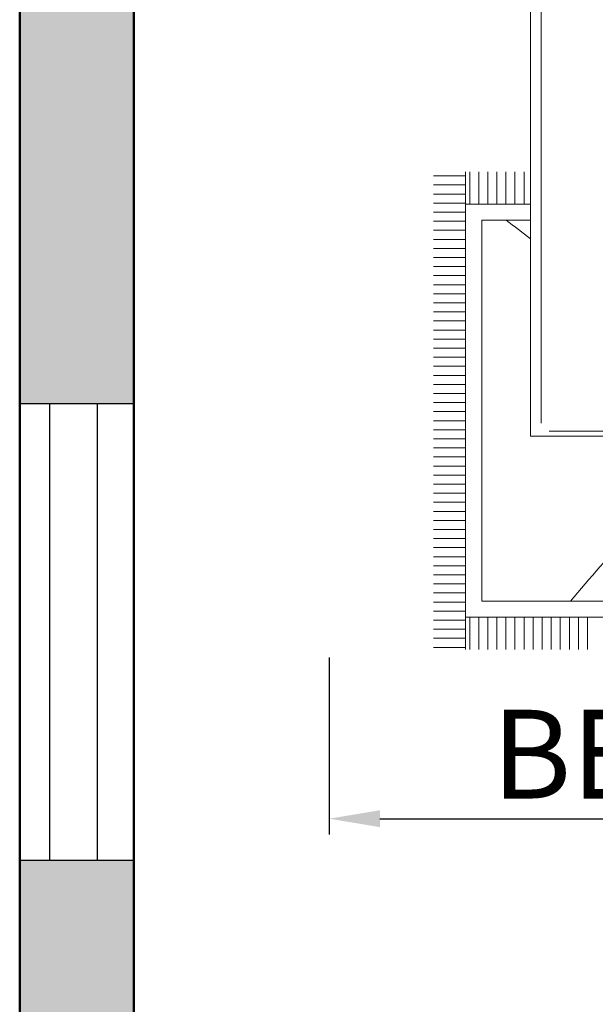
# Model space of a CAD drawing. Units: inches. Extents: x -7 to 1228, y -146 to 1091.
# Tile 8 of 88: x 60 to 105, y 375 to 453. Entities that reach past the tile are written whole.
import ezdxf

# ---------------------------------------------------------------- set-up
doc = ezdxf.new("R2010")
doc.units = ezdxf.units.IN
for name, color, linetype, lineweight in [('A-ANNO-DIMS', 2, 'Continuous', 18), ('A-FURN', 8, 'Continuous', 18), ('A-GLAZ', 175, 'Continuous', 25), ('A-WALL', 7, 'Continuous', 50), ('A-WALL-PATT', 251, 'Continuous', 13)]:
    doc.layers.add(name, color=color, linetype=linetype, lineweight=lineweight)
doc.styles.add('DIM_FONT', font='SIMPLEX.shx', dxfattribs={"width": 0.8})
doc.styles.get("Standard").update_dxf_attribs({"font": 'arial.ttf'})
doc.dimstyles.new('ISO-25', dxfattribs={"dimtxt": 7, "dimasz": 4, "dimexe": 1.25, "dimexo": 0.625, "dimtad": 1, "dimdec": 1, "dimlunit": 3, "dimtxsty": 'Standard', "dimcen": 2.5, "dimadec": 0, "dimazin": 0, "dimtfac": 1, "dimtdec": 1, "dimtmove": 1, "dimatfit": 3, "dimfxl": 1, "dimarcsym": 0})

# ---------------------------------------------------------------- blocks, each defined once
blk = doc.blocks.new('A$C4F634EDD')
for p, q in [((0.5, 0.5295), (0.5, 2.6295)), ((0.5258, 2.121), (0.5258, 0.5617)), ((0.2586, 1.1753), (0.3386, 1.1753)), ((0.3386, 0), (0.3386, 1.1852)), ((0.3486, 1.1052), (0.3486, 1.1852)), ((0.3711, 1.1052), (0.3711, 1.1852)), ((0.3936, 1.1052), (0.3936, 1.1852)), ((0.4161, 1.1052), (0.4161, 1.1852)), ((0.4386, 1.1052), (0.4386, 1.1852)), ((0.4611, 1.1052), (0.4611, 1.1852)), ((0.4836, 1.1052), (0.4836, 1.1852)), ((0.2586, 1.1528), (0.3386, 1.1528)), ((0.2586, 1.1303), (0.3386, 1.1303)), ((0.2586, 1.1078), (0.3386, 1.1078)), ((0.3386, 1.1052), (0.5, 1.1052)), ((0.2586, 1.0853), (0.3386, 1.0853)), ((0.2586, 1.0628), (0.3386, 1.0628)), ((0.3786, 1.0652), (0.5, 1.0652)), ((0.3786, 0.12), (0.3786, 1.0652)), ((0.2586, 1.0403), (0.3386, 1.0403)), ((0.2586, 1.0178), (0.3386, 1.0178)), ((0.2586, 0.9953), (0.3386, 0.9953)), ((0.2586, 0.9728), (0.3386, 0.9728)), ((0.2586, 0.9503), (0.3386, 0.9503)), ((0.2586, 0.9278), (0.3386, 0.9278)), ((0.2586, 0.9053), (0.3386, 0.9053)), ((0.2586, 0.8828), (0.3386, 0.8828)), ((0.2586, 0.8603), (0.3386, 0.8603)), ((0.2586, 0.8378), (0.3386, 0.8378)), ((0.2586, 0.8153), (0.3386, 0.8153)), ((0.2586, 0.7928), (0.3386, 0.7928)), ((0.2586, 0.7703), (0.3386, 0.7703)), ((0.2586, 0.7478), (0.3386, 0.7478)), ((0.2586, 0.7253), (0.3386, 0.7253)), ((0.2586, 0.7028), (0.3386, 0.7028)), ((0.2586, 0.6803), (0.3386, 0.6803)), ((0.2586, 0.6578), (0.3386, 0.6578)), ((0.2586, 0.6353), (0.3386, 0.6353)), ((0.2586, 0.6128), (0.3386, 0.6128)), ((0.2586, 0.5903), (0.3386, 0.5903)), ((0.2586, 0.5678), (0.3386, 0.5678)), ((0.2586, 0.5453), (0.3386, 0.5453)), ((0.5458, 0.5417), (2.2516, 0.5417)), ((0.2586, 0.5228), (0.3386, 0.5228)), ((2.3, 0.5295), (0.5, 0.5295)), ((0.2586, 0.5003), (0.3386, 0.5003)), ((0.2586, 0.4778), (0.3386, 0.4778)), ((0.2586, 0.4553), (0.3386, 0.4553)), ((0.2586, 0.4328), (0.3386, 0.4328)), ((0.2586, 0.4103), (0.3386, 0.4103)), ((0.2586, 0.3878), (0.3386, 0.3878)), ((0.2586, 0.3653), (0.3386, 0.3653)), ((0.2586, 0.3428), (0.3386, 0.3428)), ((0.2586, 0.3203), (0.3386, 0.3203)), ((0.2586, 0.2978), (0.3386, 0.2978)), ((0.2586, 0.2753), (0.3386, 0.2753)), ((0.2586, 0.2528), (0.3386, 0.2528)), ((0.2586, 0.2303), (0.3386, 0.2303)), ((0.2586, 0.2078), (0.3386, 0.2078)), ((0.2586, 0.1853), (0.3386, 0.1853)), ((0.2586, 0.1628), (0.3386, 0.1628)), ((0.2586, 0.1403), (0.3386, 0.1403)), ((0.2586, 0.1178), (0.3386, 0.1178)), ((2.4188, 0.12), (0.3786, 0.12)), ((0.2586, 0.0953), (0.3386, 0.0953)), ((2.4588, 0.08), (0.3386, 0.08)), ((0.3486, 0), (0.3486, 0.08)), ((0.3711, 0), (0.3711, 0.08)), ((0.3936, 0), (0.3936, 0.08)), ((0.4161, 0), (0.4161, 0.08)), ((0.4386, 0), (0.4386, 0.08)), ((0.4611, 0), (0.4611, 0.08)), ((0.4836, 0), (0.4836, 0.08)), ((0.5061, 0), (0.5061, 0.08)), ((0.5286, 0), (0.5286, 0.08)), ((0.5511, 0), (0.5511, 0.08)), ((0.5736, 0), (0.5736, 0.08)), ((0.5961, 0), (0.5961, 0.08)), ((0.6186, 0), (0.6186, 0.08)), ((0.6411, 0), (0.6411, 0.08)), ((0.2586, 0.0728), (0.3386, 0.0728)), ((0.2586, 0.0503), (0.3386, 0.0503)), ((0.2586, 0.0278), (0.3386, 0.0278)), ((0.2586, 0.0053), (0.3386, 0.0053))]:
    blk.add_line(p, q)
blk.add_open_spline([(0.4393, 1.0652), (0.4595, 1.05), (0.4798, 1.0348), (0.5, 1.0195)], degree=3)
blk.add_open_spline([(0.5992, 0.12), (0.6957, 0.2341), (0.8523, 0.4189), (1.0536, 0.5069), (1.136, 0.5295)], degree=3, knots=[0, 0, 0, 0, 432.822832, 701.445452, 701.445452, 701.445452, 701.445452])
at = {"style": 'DIM_FONT', "width": 0.8, "flags": 9}
for tag, p in [('YSIZE', (0.5, 2.6295)), ('XSIZE', (0.5, 2.6295)), ('XSIZE', (2.2985, 2.6295)), ('YSIZE', (2.2985, 2.6295))]:
    blk.add_attdef(tag, p, '', height=0.0005, dxfattribs=at)
blk = doc.blocks.new('WIN-36')
for p, q in [((0, 36), (0, 0)), ((9, 36), (0, 36)), ((2.343, 36), (2.343, 0)), ((6.137, 0), (6.137, 36)), ((9, 0), (9, 36)), ((0, 0), (9, 0)), ((2.343, 0), (6.137, 0))]:
    blk.add_line(p, q)
blk = doc.blocks.new('*D24')
at = {"layer": 'A-ANNO-DIMS', "color": 0, "lineweight": -2, "transparency": 16777216}
for p, q in [((84.435, 402.798), (84.435, 388.824)), ((173.431, 402.798), (173.431, 388.824)), ((88.435, 390.074), (169.431, 390.074))]:
    blk.add_line(p, q, dxfattribs=at)
at = {"layer": 'A-ANNO-DIMS', "color": 0, "transparency": 16777216}
for points in [[(88.435, 390.741), (88.435, 389.407), (84.435, 390.074)], [(169.431, 390.741), (169.431, 389.407), (173.431, 390.074)]]:
    blk.add_solid(points, dxfattribs=at)
at = {"layer": 'Defpoints', "color": 0, "transparency": 16777216}
for p in [(84.435, 403.423), (173.431, 403.423), (173.431, 390.074)]:
    blk.add_point(p, dxfattribs=at)
at = {"layer": 'A-ANNO-DIMS', "color": 0, "transparency": 16777216, "insert": (128.933, 394.259), "char_height": 7, "attachment_point": 5}
blk.add_mtext('BED 7\'-5" TYP.', dxfattribs=at)

msp = doc.modelspace()

# ---------------------------------------------------------------- hatches: boundary and pattern name
at = {"layer": 'A-WALL-PATT'}
h = msp.add_hatch(color=256, dxfattribs=at)
h.dxf.hatch_style = 1
h.paths.add_polyline_path([(69, 568), (60, 568), (60, 493), (63.289, 493), (69, 493)])
h.paths.add_polyline_path([(69, 662.405), (60, 662.405), (60, 586), (69, 586)], flags=17)
h.paths.add_polyline_path([(69, 723), (184, 723), (184, 734), (179, 734), (179, 728), (69, 728), (69, 741.623), (60, 741.623), (60, 698.405), (69, 698.405)], flags=17)
h.paths.add_polyline_path([(69, 782), (231, 782), (231, 728), (231, 723), (231, 586), (236, 586), (236, 787), (69, 787), (69, 800.126), (60, 800.126), (60, 765.623), (69, 765.623)])
h.paths.add_polyline_path([(184, 842), (189, 842), (189, 848), (173, 848), (173, 842), (179, 842), (179, 787), (184, 787)])
h.paths.add_polyline_path([(118.22, 69), (69, 69), (69, 60), (118.22, 60)])
h.paths.add_polyline_path([(227, 69), (154.22, 69), (154.22, 60), (227, 60)])
h.paths.add_polyline_path([(236, 60), (232.711, 60), (227, 60), (227, 36), (236, 36)])
h.paths.add_polyline_path([(389, 60), (380, 60), (380, 36), (389, 36)])
h.paths.add_polyline_path([(384, 181), (380, 181), (380, 115), (380, 78), (384, 78)])
h.paths.add_polyline_path([(380, 115), (334.547, 115), (334.547, 109), (380, 109)])
h.paths.add_polyline_path([(274.547, 115), (236, 115), (236, 201), (232.711, 201), (231, 201), (231, 78), (236, 78), (236, 109), (274.547, 109)])
h.paths.add_polyline_path([(69, 123), (60, 123), (60, 78), (69, 78)])
h.paths.add_polyline_path([(69, 201), (60, 201), (60, 159), (69, 159)])
h.paths.add_polyline_path([(143, 219), (69, 219), (69, 213), (143, 213)], flags=17)
h.paths.add_polyline_path([(189, 219), (184, 219), (184, 274), (231, 274), (231, 219), (236, 219), (236, 279), (184, 279), (184, 297), (179, 297), (179, 279), (69, 279), (69, 290.912), (60, 290.912), (60, 262.179), (69, 262.179), (69, 274), (179, 274), (179, 219), (173, 219), (173, 213), (189, 213)])
h.paths.add_polyline_path([(69, 238.179), (60, 238.179), (60, 219), (69, 219)], flags=17)
h.paths.add_polyline_path([(69, 333), (60, 333), (60, 314.912), (69, 314.912), (69, 316.965)])
h.paths.add_polyline_path([(190, 338), (184, 338), (69, 338), (69, 333), (179, 333), (179, 327), (184, 327), (184, 333.021), (190, 333.046)])
h.paths.add_polyline_path([(69, 386.806), (60, 386.806), (60, 351), (69, 351)])
h.paths.add_polyline_path([(69, 475), (60, 475), (60, 422.806), (69, 422.806)])
h.paths.add_polyline_path([(236, 475), (231, 475), (231, 351.238), (236, 351.238)])
h.paths.add_polyline_path([(384, 475), (380, 475), (380, 362), (384, 362)])
h.paths.add_polyline_path([(547, 307), (439, 307), (439, 356), (445, 356), (445, 362), (433, 362), (433, 307), (380, 307), (380, 244), (380, 241), (384, 241), (384, 301), (433, 301), (433, 277), (439, 277), (439, 301), (547, 301)])
h.paths.add_polyline_path([(547, 241), (439, 241), (439, 247), (433, 247), (433, 235), (547, 235)])
h.paths.add_polyline_path([(450, 69), (440.286, 69), (424.889, 69), (389, 69), (389, 60), (450, 60)])
h.paths.add_polyline_path([(547, 69), (486, 69), (486, 60), (547, 60)])
h.paths.add_polyline_path([(556, 148.268), (547, 148.268), (547, 78), (556, 78)])
h.paths.add_polyline_path([(556, 223), (547, 223), (547, 195), (547, 184.268), (556, 184.268)])
h.paths.add_polyline_path([(556, 311.192), (547, 311.192), (547, 273.075), (556, 273.075)])
h.paths.add_polyline_path([(556, 344), (552.711, 344), (547, 344), (547, 335.192), (556, 335.192)])
h.paths.add_polyline_path([(556, 249.075), (547, 249.075), (547, 241), (556, 241)])
h.paths.add_polyline_path([(547, 362), (475, 362), (475, 356), (547, 356)], flags=0)
h.paths.add_polyline_path([(556, 399.621), (547, 399.621), (547, 362), (556, 362)])
h.paths.add_polyline_path([(556, 475), (547, 475), (547, 435.621), (556, 435.621)])
h.paths.add_polyline_path([(547, 493), (389, 493), (389, 487), (547, 487)])
h.paths.add_polyline_path([(380, 493), (278, 493), (278, 487), (380, 487)])
h.paths.add_polyline_path([(227, 493), (69, 493), (69, 487), (227, 487)])
h.paths.add_polyline_path([(643, 122.445), (634, 122.445), (634, 78), (643, 78)])
h.paths.add_polyline_path([(702.5, 69), (692.786, 69), (677.389, 69), (643, 69), (643, 60), (702.5, 60)])
h.paths.add_polyline_path([(798, 69), (738.5, 69), (738.5, 60), (798, 60)])
h.paths.add_polyline_path([(807, 60), (803.711, 60), (798, 60), (798, 36), (807, 36)])
h.paths.add_polyline_path([(807, 109), (846.751, 109), (846.751, 115), (807, 115), (807, 159), (802, 159), (802, 78), (807, 78)])
h.paths.add_polyline_path([(807, 201), (802, 201), (802, 195), (807, 195)])
h.paths.add_polyline_path([(643, 201), (634, 201), (634, 158.445), (643, 158.445)])
h.paths.add_polyline_path([(756, 225), (751, 225), (751, 219), (643, 219), (643, 213), (756, 213)])
h.paths.add_polyline_path([(643, 240.848), (634, 240.848), (634, 219), (643, 219)])
h.paths.add_polyline_path([(643, 274), (643, 288.629), (634, 288.629), (634, 264.848), (643, 264.848)])
h.paths.add_polyline_path([(802, 279), (756, 279), (756, 297), (751, 297), (751, 279), (643, 279), (643, 274), (751, 274), (751, 255), (756, 255), (756, 274), (802, 274)])
h.paths.add_polyline_path([(807, 333), (803.711, 333), (802, 333), (802, 279), (802, 274), (802, 219), (807, 219)])
h.paths.add_polyline_path([(956, 182), (951, 182), (951, 115), (906.751, 115), (906.751, 109), (951, 109), (951, 78), (956, 78)])
h.paths.add_polyline_path([(960, 60), (951, 60), (951, 36), (960, 36)])
h.paths.add_polyline_path([(1021, 69), (1005.781, 69), (960, 69), (960, 60), (1021, 60)])
h.paths.add_polyline_path([(956, 224), (951, 224), (951, 218), (956, 218)])
h.paths.add_polyline_path([(956, 302), (1004, 302), (1004, 278), (1010, 278), (1010, 302), (1118, 302), (1118, 290.809), (1127, 290.809), (1127, 326.968), (1118, 326.968), (1118, 320.966), (1118, 307), (1010, 307), (1010, 356), (1016, 356), (1016, 362), (1004, 362), (1004, 307), (951, 307), (951, 244), (951, 242), (954.289, 242), (956, 242)])
h.paths.add_polyline_path([(643, 333), (634, 333), (634, 312.629), (643, 312.629), (643, 316.965)])
h.paths.add_polyline_path([(756, 338), (643, 338), (643, 333), (751, 333), (751, 327), (756, 327)])
h.paths.add_polyline_path([(643, 388), (634, 388), (634, 351), (643, 351)])
h.paths.add_polyline_path([(807, 357), (802, 357), (802, 351), (807, 351)])
h.paths.add_polyline_path([(807, 475), (802, 475), (802, 393), (807, 393)])
h.paths.add_polyline_path([(643, 475), (634, 475), (634, 424), (643, 424)])
h.paths.add_polyline_path([(798, 493), (643, 493), (643, 487), (798, 487)])
h.paths.add_polyline_path([(634, 493), (556, 493), (556, 487), (634, 487)])
h.paths.add_polyline_path([(813, 493), (807, 493), (807, 487), (813, 487)])
h.paths.add_polyline_path([(951, 493), (849, 493), (849, 487), (951, 487)])
h.paths.add_polyline_path([(956, 484), (951, 484), (951, 374), (956, 374)])
h.paths.add_polyline_path([(1109, 493), (969, 493), (969, 487), (1109, 487)])
h.paths.add_polyline_path([(1127, 484), (1118, 484), (1118, 450.641), (1127, 450.641)])
h.paths.add_polyline_path([(1127, 414.641), (1118, 414.641), (1118, 365), (1127, 365)])
h.paths.add_polyline_path([(1109, 362), (1046, 362), (1046, 356), (1109, 356)], flags=17)
h.paths.add_polyline_path([(1127, 356), (1123.454, 356), (1118, 356), (1118, 350.968), (1127, 350.968)], flags=0)
h.paths.add_polyline_path([(1127, 266.809), (1118, 266.809), (1118, 262.361), (1118, 242), (1127, 242)], flags=17)
h.paths.add_polyline_path([(1118, 242), (1010, 242), (1010, 248), (1004, 248), (1004, 237), (1118, 237)])
h.paths.add_polyline_path([(1127, 224), (1118, 224), (1118, 170), (1127, 170)])
h.paths.add_polyline_path([(1127, 134), (1118, 134), (1118, 78), (1127, 78)])
h.paths.add_polyline_path([(1118, 69), (1057, 69), (1057, 60), (1118, 60)])
h.paths.add_polyline_path([(227, 571.546), (227, 574), (69, 574), (69, 568), (227, 568)])
h.paths.add_polyline_path([(380, 571.546), (380, 574), (278, 574), (278, 568), (380, 568)])
h.paths.add_polyline_path([(242, 574), (236, 574), (236, 568), (242, 568)])
h.paths.add_polyline_path([(547, 571.546), (547, 574), (389, 574), (389, 568), (547, 568)])
h.paths.add_polyline_path([(384, 733), (380, 733), (380, 586), (384, 586)])
h.paths.add_polyline_path([(556, 646), (634, 646), (634, 655), (547, 655), (547, 586), (556, 586)])
h.paths.add_polyline_path([(634, 574), (556, 574), (556, 568), (634, 568)])
h.paths.add_polyline_path([(643, 655), (634, 655), (634, 586), (643, 586)])
h.paths.add_polyline_path([(798, 574), (643, 574), (643, 568), (798, 568)])
h.paths.add_polyline_path([(643, 663.854), (634, 663.854), (634, 655), (643, 655)])
h.paths.add_polyline_path([(556, 676.967), (547, 676.967), (547, 655), (556, 655)])
h.paths.add_polyline_path([(556, 733), (547, 733), (547, 712.967), (556, 712.967)])
h.paths.add_polyline_path([(643, 710), (634, 710), (634, 699.854), (643, 699.854)])
h.paths.add_polyline_path([(807, 668), (802, 668), (802, 586), (807, 586)])
h.paths.add_polyline_path([(951, 574), (849, 574), (849, 568), (951, 568)])
h.paths.add_polyline_path([(956, 691), (951, 691), (951, 577), (956, 577)])
h.paths.add_polyline_path([(1109, 574), (969, 574), (969, 568), (1109, 568)])
h.paths.add_polyline_path([(1127, 643.403), (1118, 643.403), (1118, 577), (1127, 577)])
h.paths.add_polyline_path([(1127, 568), (1123.454, 568), (1118, 568), (1118, 493), (1127, 493)])
h.paths.add_polyline_path([(1127, 733), (1118, 733), (1118, 679.403), (1127, 679.403)])
h.paths.add_polyline_path([(1127, 777.348), (1118, 777.348), (1118, 770.035), (1118, 751), (1127, 751)], flags=17)
h.paths.add_polyline_path([(1118, 751), (1010, 751), (1010, 757), (1004, 757), (1004, 745), (1118, 745)])
h.paths.add_polyline_path([(956, 811), (1004, 811), (1004, 787), (1010, 787), (1010, 811), (1017.874, 811), (1017.874, 811.627, -0.414214), (1018.247, 812), (1031.978, 812, -0.414214), (1032.351, 811.627), (1032.351, 811), (1118, 811), (1118, 801.348), (1127, 801.348), (1127, 834.685), (1118, 834.685), (1118, 830.238), (1118, 817), (1010, 817), (1010, 866), (1016, 866), (1016, 872), (1004, 872), (1004, 817), (956, 817), (956, 866), (951, 866), (951, 751), (954.289, 751), (956, 751)])
h.paths.add_polyline_path([(1118, 872), (1046, 872), (1046, 866), (1118, 866)], flags=17)
h.paths.add_polyline_path([(1127, 924.711), (1118, 924.711), (1118, 884), (1127, 884)])
h.paths.add_polyline_path([(1127, 866), (1123.711, 866), (1118, 866), (1118, 858.685), (1127, 858.685)], flags=17)
h.paths.add_polyline_path([(956, 983), (951, 983), (951, 952), (807, 952), (807, 983), (802, 983), (802, 902), (807, 902), (807, 946), (951, 946), (951, 884), (956, 884)])
h.paths.add_polyline_path([(807, 842), (802, 842), (802, 787), (756, 787), (756, 806), (751, 806), (751, 787), (643, 787), (643, 782), (751, 782), (751, 764), (756, 764), (756, 782), (802, 782), (802, 728), (807, 728)])
h.paths.add_polyline_path([(756, 848), (643, 848), (643, 842), (751, 842), (751, 836), (756, 836)])
h.paths.add_polyline_path([(756, 734), (751, 734), (751, 728), (643, 728), (643, 723), (756, 723)])
h.paths.add_polyline_path([(643, 749.791), (634, 749.791), (634, 728), (637.289, 728), (643, 728)])
h.paths.add_polyline_path([(643, 805.405), (634, 805.405), (634, 773.791), (643, 773.791)])
h.paths.add_polyline_path([(643, 896.663), (634, 896.663), (634, 860), (637.289, 860), (643, 860)])
h.paths.add_polyline_path([(643, 842), (634, 842), (634, 829.405), (643, 829.405)])
h.paths.add_polyline_path([(643, 983), (634, 983), (634, 932.663), (643, 932.663)])
h.paths.add_polyline_path([(1127, 983), (1118, 983), (1118, 960.711), (1127, 960.711)])
h.paths.add_polyline_path([(1118, 1001), (1077.525, 1001), (1077.525, 992), (1118, 992)])
h.paths.add_polyline_path([(1041.525, 1001), (960, 1001), (960, 992), (1041.525, 992)])
h.paths.add_polyline_path([(960, 1025), (951, 1025), (951, 1001), (954.289, 1001), (960, 1001)])
h.paths.add_polyline_path([(807, 1025), (798, 1025), (798, 1001), (807, 1001)])
h.paths.add_polyline_path([(798, 1001), (738.5, 1001), (738.5, 992), (798, 992)])
h.paths.add_polyline_path([(702.5, 1001), (643, 1001), (643, 992), (702.5, 992)])
h.paths.add_polyline_path([(547, 1001), (499.113, 1001), (499.113, 992), (547, 992)])
h.paths.add_polyline_path([(463.113, 1001), (389, 1001), (389, 992), (463.113, 992)])
h.paths.add_polyline_path([(389, 1025), (380, 1025), (380, 1022), (380, 1001), (383.289, 1001), (389, 1001)])
h.paths.add_polyline_path([(236, 1025), (227, 1025), (227, 1001), (236, 1001)])
h.paths.add_polyline_path([(236, 983), (231, 983), (231, 860), (236, 860)])
h.paths.add_polyline_path([(274.547, 952), (236, 952), (236, 946), (274.547, 946)])
h.paths.add_polyline_path([(380, 952), (334.547, 952), (334.547, 946), (380, 946)])
h.paths.add_polyline_path([(384, 983), (380, 983), (380, 884), (383.289, 884), (384, 884)])
h.paths.add_polyline_path([(227, 1001), (155.012, 1001), (155.012, 992), (162.875, 992), (227, 992)])
h.paths.add_polyline_path([(119.012, 1001), (69, 1001), (69, 992), (119.012, 992)])
h.paths.add_polyline_path([(69, 983), (60, 983), (60, 922.987), (69, 922.987)])
h.paths.add_polyline_path([(69, 886.987), (60, 886.987), (60, 860), (63.289, 860), (69, 860)])
h.paths.add_polyline_path([(143, 848), (69, 848), (69, 842), (143, 842)])

# ---------------------------------------------------------------- linework, layer by layer
at = {"layer": 'A-WALL'}
for p, q in [((60, 1001), (60, 60)), ((69, 568), (69, 279)), ((69, 338), (69, 487))]:
    msp.add_line(p, q, dxfattribs=at)

# ---------------------------------------------------------------- block references
at = {"layer": 'A-FURN', "xscale": 31.78426361944092, "yscale": 31.78426361944092, "zscale": 31.78426361944092}
msp.add_blockref('A$C4F634EDD', (84.435, 403.423), dxfattribs=at)
at = {"layer": 'A-GLAZ'}
msp.add_blockref('WIN-36', (60, 386.806), dxfattribs=at)

# ---------------------------------------------------------------- dimensions: what is measured, and where the dimension line sits
at = {"layer": 'A-ANNO-DIMS'}
dim = msp.add_linear_dim(base=(173.431, 390.074), p1=(84.435, 403.423), p2=(173.431, 403.423), text='BED <> TYP.', dimstyle='ISO-25', override={"dimdec": 1, "dimlfac": 1, "dimrnd": 0, "dimzin": 1, "dimdsep": 46, "dimlunit": 4, "dimfrac": 2}, dxfattribs=at)
dim.commit()
dim.dimension.update_dxf_attribs({"geometry": '*D24', "text_midpoint": (128.933, 394.259)})

doc.saveas('drawing.dxf')
